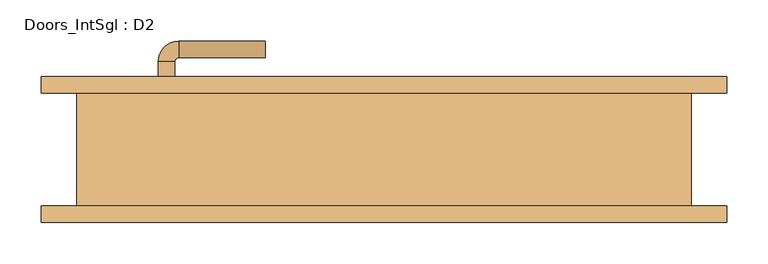
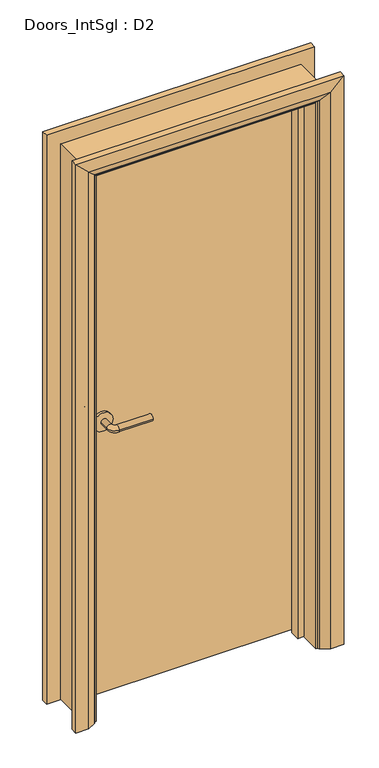
"""IFC4 building model written with IfcOpenShell, lengths in millimetres: door geometry, Doors_IntSgl : D2."""

from ifc_helpers import new_model, si_unit, point, frame, frame_2d, origin, place, context, project, spatial, polyline, circle_curve, ellipse_curve, trimmed, segment, composite_curve, outline, extrude, faceted_brep, source, transform, mapped, element, save
from ifc_brep_helpers import plane_surface, cylinder_surface, revolved_surface, advanced_brep


def doors_intsgl_d2_4a296642(model_context):
    return source(origin(), model_context, "Body", "SolidModel", [
        advanced_brep(
        [(-274.0, 22.58, 900.0), (-254.0, 22.58, 900.0), (-254.0, -7.42, 900.0), (-274.0, -7.42, 900.0), (-249.0, -12.42, 900.0), (-249.0, -32.42, 900.0), (-144.0, -32.42, 900.0), (-144.0, -12.42, 900.0)],
        [
            (0, 1, circle_curve(frame((-264.0, 22.58, 900.0), z_axis=(0.0, 1.0, 0.0), x_axis=(1.0, 0.0, 0.0)), 10.0)),
            (1, 0, circle_curve(frame((-264.0, 22.58, 900.0), z_axis=(0.0, 1.0, 0.0), x_axis=(1.0, 0.0, 0.0)), 10.0)),
            (1, 2),
            (2, 3, circle_curve(frame((-264.0, -7.42, 900.0), z_axis=(0.0, 1.0, 0.0), x_axis=(1.0, 0.0, 0.0)), 10.0)),
            (3, 0),
            (3, 2, circle_curve(frame((-264.0, -7.42, 900.0), z_axis=(0.0, 1.0, 0.0), x_axis=(1.0, 0.0, 0.0)), 10.0)),
            (4, 5, circle_curve(frame((-249.0, -22.42, 900.0), z_axis=(-1.0, 0.0, 0.0), x_axis=(0.0, 1.0, 0.0)), 10.0)),
            (5, 3, circle_curve(frame((-249.0, -7.42, 900.0), z_axis=(0.0, 0.0, -1.0), x_axis=(-1.0, 0.0, 0.0)), 25.0)),
            (2, 4, circle_curve(frame((-249.0, -7.42, 900.0), z_axis=(0.0, 0.0, 1.0), x_axis=(-1.0, 0.0, 0.0)), 5.0)),
            (5, 4, circle_curve(frame((-249.0, -22.42, 900.0), z_axis=(-1.0, 0.0, 0.0), x_axis=(0.0, 1.0, 0.0)), 10.0)),
            (6, 7, circle_curve(frame((-144.0, -22.42, 900.0), z_axis=(1.0, 0.0, 0.0), x_axis=(0.0, 1.0, 0.0)), 10.0)),
            (7, 6, circle_curve(frame((-144.0, -22.42, 900.0), z_axis=(1.0, 0.0, 0.0), x_axis=(0.0, 1.0, 0.0)), 10.0)),
            (4, 7),
            (6, 5),
        ],
        [
            plane_surface(frame((-264.0, 22.58, 900.0), z_axis=(0.0, 1.0, 0.0), x_axis=(0.0, 0.0, 1.0))),
            cylinder_surface(frame((-264.0, 22.58, 900.0), z_axis=(0.0, 1.0, 0.0), x_axis=(1.0, 0.0, 0.0)), 10.0),
            revolved_surface(trimmed(ellipse_curve(frame((-264.0, -7.42, 900.0), z_axis=(0.0, -1.0, 0.0), x_axis=(1.0, 0.0, 0.0)), 10.0, 10.0), [point((-274.0, -7.42, 900.0))], [point((-254.0, -7.42, 900.0))], True, "CARTESIAN"), (-249.0, -7.42, 900.0), (0.0, 0.0, -1.0)),
            revolved_surface(trimmed(ellipse_curve(frame((-264.0, -7.42, 900.0), z_axis=(0.0, -1.0, 0.0), x_axis=(1.0, 0.0, 0.0)), 10.0, 10.0), [point((-254.0, -7.42, 900.0))], [point((-274.0, -7.42, 900.0))], True, "CARTESIAN"), (-249.0, -7.42, 900.0), (0.0, 0.0, -1.0)),
            plane_surface(frame((-144.0, -22.42, 900.0), z_axis=(1.0, 0.0, 0.0), x_axis=(0.0, 0.0, 1.0))),
            cylinder_surface(frame((-249.0, -22.42, 900.0), z_axis=(-1.0, 0.0, 0.0), x_axis=(0.0, 1.0, 0.0)), 10.0),
        ],
        [
            (0, [[1, 2]]),
            (1, [[3, 4, 5, -2]]),
            (1, [[-5, 6, -3, -1]]),
            (2, [[7, 8, -4, 9]]),
            (3, [[10, -9, -6, -8]]),
            (4, [[11, 12]]),
            (5, [[13, -11, 14, -7]]),
            (5, [[-14, -12, -13, -10]]),
        ],
    ),
        extrude(outline(composite_curve([segment(trimmed(circle_curve(frame_2d((900.0, -266.5)), 30.0), [point((900.0, -296.5))], [point((900.0, -236.5))], False, "CARTESIAN"), True, "CONTINUOUS"), segment(trimmed(circle_curve(frame_2d((900.0, -266.5)), 30.0), [point((900.0, -236.5))], [point((900.0, -296.5))], False, "CARTESIAN"), True, "CONTINUOUS")], self_intersect=False)), frame((0.0, 22.58, 0.0), z_axis=(0.0, 1.0, 0.0), x_axis=(0.0, 0.0, 1.0)), (0.0, 0.0, 1.0), 8.0),
        advanced_brep(
        [(-274.0, 76.58, 900.0), (-254.0, 76.58, 900.0), (-274.0, 106.58, 900.0), (-254.0, 106.58, 900.0), (-249.0, 111.58, 900.0), (-249.0, 131.58, 900.0), (-144.0, 131.58, 900.0), (-144.0, 111.58, 900.0)],
        [
            (0, 1, circle_curve(frame((-264.0, 76.58, 900.0), z_axis=(0.0, -1.0, 0.0), x_axis=(1.0, 0.0, 0.0)), 10.0)),
            (1, 0, circle_curve(frame((-264.0, 76.58, 900.0), z_axis=(0.0, -1.0, 0.0), x_axis=(1.0, 0.0, 0.0)), 10.0)),
            (0, 2),
            (2, 3, circle_curve(frame((-264.0, 106.58, 900.0), z_axis=(0.0, -1.0, 0.0), x_axis=(1.0, 0.0, 0.0)), 10.0)),
            (3, 1),
            (3, 2, circle_curve(frame((-264.0, 106.58, 900.0), z_axis=(0.0, -1.0, 0.0), x_axis=(1.0, 0.0, 0.0)), 10.0)),
            (4, 3, circle_curve(frame((-249.0, 106.58, 900.0), z_axis=(0.0, 0.0, 1.0), x_axis=(-1.0, 0.0, 0.0)), 5.0)),
            (2, 5, circle_curve(frame((-249.0, 106.58, 900.0), z_axis=(0.0, 0.0, -1.0), x_axis=(-1.0, 0.0, 0.0)), 25.0)),
            (5, 4, circle_curve(frame((-249.0, 121.58, 900.0), z_axis=(-1.0, 0.0, 0.0), x_axis=(0.0, -1.0, 0.0)), 10.0)),
            (4, 5, circle_curve(frame((-249.0, 121.58, 900.0), z_axis=(-1.0, 0.0, 0.0), x_axis=(0.0, -1.0, 0.0)), 10.0)),
            (6, 7, circle_curve(frame((-144.0, 121.58, 900.0), z_axis=(1.0, 0.0, 0.0), x_axis=(0.0, -1.0, 0.0)), 10.0)),
            (7, 6, circle_curve(frame((-144.0, 121.58, 900.0), z_axis=(1.0, 0.0, 0.0), x_axis=(0.0, -1.0, 0.0)), 10.0)),
            (5, 6),
            (7, 4),
        ],
        [
            plane_surface(frame((-264.0, 76.58, 900.0), z_axis=(0.0, -1.0, 0.0), x_axis=(0.0, 0.0, 1.0))),
            cylinder_surface(frame((-264.0, 76.58, 900.0), z_axis=(0.0, -1.0, 0.0), x_axis=(1.0, 0.0, 0.0)), 10.0),
            revolved_surface(trimmed(ellipse_curve(frame((-264.0, 106.58, 900.0), z_axis=(0.0, -1.0, 0.0), x_axis=(1.0, 0.0, 0.0)), 10.0, 10.0), [point((-274.0, 106.58, 900.0))], [point((-254.0, 106.58, 900.0))], True, "CARTESIAN"), (-249.0, 106.58, 900.0), (0.0, 0.0, -1.0)),
            revolved_surface(trimmed(ellipse_curve(frame((-264.0, 106.58, 900.0), z_axis=(0.0, -1.0, 0.0), x_axis=(1.0, 0.0, 0.0)), 10.0, 10.0), [point((-254.0, 106.58, 900.0))], [point((-274.0, 106.58, 900.0))], True, "CARTESIAN"), (-249.0, 106.58, 900.0), (0.0, 0.0, -1.0)),
            plane_surface(frame((-144.0, 121.58, 900.0), z_axis=(1.0, 0.0, 0.0), x_axis=(0.0, 0.0, 1.0))),
            cylinder_surface(frame((-249.0, 121.58, 900.0), z_axis=(-1.0, 0.0, 0.0), x_axis=(0.0, -1.0, 0.0)), 10.0),
        ],
        [
            (0, [[1, 2]]),
            (1, [[-1, 3, 4, 5]]),
            (1, [[-2, -5, 6, -3]]),
            (2, [[7, -4, 8, 9]]),
            (3, [[-8, -6, -7, 10]]),
            (4, [[11, 12]]),
            (5, [[-9, 13, -12, 14]]),
            (5, [[-10, -14, -11, -13]]),
        ],
    ),
        extrude(outline(composite_curve([segment(trimmed(circle_curve(frame_2d((900.0, -266.5)), 30.0), [point((900.0, -296.5))], [point((900.0, -236.5))], False, "CARTESIAN"), True, "CONTINUOUS"), segment(trimmed(circle_curve(frame_2d((900.0, -266.5)), 30.0), [point((900.0, -236.5))], [point((900.0, -296.5))], False, "CARTESIAN"), True, "CONTINUOUS")], self_intersect=False)), frame((0.0, 68.58, 0.0), z_axis=(0.0, 1.0, 0.0), x_axis=(0.0, 0.0, 1.0)), (0.0, 0.0, 1.0), 8.0),
        extrude(outline(polyline([(339.0, 30.58), (-339.0, 30.58), (-339.0, 68.58), (339.0, 68.58), (339.0, 30.58)])), frame((0.0, 0.0, 8.0), z_axis=(0.0, 0.0, 1.0), x_axis=(1.0, 0.0, 0.0)), (0.0, 0.0, 1.0), 1778.8),
        advanced_brep(
        [(416.0, 88.58, 0.0), (416.0, 68.58, 0.0), (346.0, 68.58, 0.0), (350.0, 74.58, 0.0), (376.0, 88.58, 0.0), (416.0, 88.58, 1863.8), (416.0, 68.58, 1863.8), (-416.0, 68.58, 1863.8), (-416.0, 68.58, 0.0), (-346.0, 68.58, 0.0), (-346.0, 68.58, 1793.8), (346.0, 68.58, 1793.8), (350.0, 74.58, 1797.8), (376.0, 88.58, 1823.8), (-376.0, 88.58, 1823.8), (-376.0, 88.58, 0.0), (-416.0, 88.58, 0.0), (-416.0, 88.58, 1863.8), (-350.0, 74.58, 0.0), (-350.0, 74.58, 1797.8)],
        [
            (0, 1),
            (1, 2),
            (2, 3, circle_curve(frame((354.0, 67.58, 0.0), z_axis=(0.0, 0.0, -1.0), x_axis=(1.0, 0.0, 0.0)), 8.0622577)),
            (3, 4),
            (4, 0),
            (0, 5),
            (5, 6),
            (6, 1),
            (6, 7),
            (7, 8),
            (8, 9),
            (9, 10),
            (10, 11),
            (11, 2),
            (11, 12, ellipse_curve(frame((354.0, 67.58, 1801.8), z_axis=(0.7071067811865475, 0.0, -0.7071067811865475), x_axis=(-0.7071067811865474, 0.0, -0.7071067811865476)), 11.4017543, 8.0622577)),
            (12, 3),
            (12, 13),
            (13, 4),
            (13, 14),
            (14, 15),
            (15, 16),
            (16, 17),
            (17, 5),
            (7, 17),
            (16, 8),
            (15, 18),
            (18, 9, circle_curve(frame((-354.0, 67.58, 0.0), z_axis=(0.0, 0.0, -1.0), x_axis=(-1.0, 0.0, 0.0)), 8.0622577)),
            (19, 10, ellipse_curve(frame((-354.0, 67.58, 1801.8), z_axis=(-0.7071067811865475, 0.0, -0.7071067811865475), x_axis=(-0.7071067811865474, 0.0, 0.7071067811865476)), 11.4017543, 8.0622577)),
            (18, 19),
            (14, 19),
            (19, 12),
        ],
        [
            plane_surface(frame((346.0, 68.58, 0.0), z_axis=(0.0, 0.0, -1.0), x_axis=(0.0, -1.0, 0.0))),
            plane_surface(frame((416.0, 88.58, 0.0), z_axis=(1.0, 0.0, 0.0), x_axis=(0.0, 0.0, 1.0))),
            plane_surface(frame((416.0, 68.58, 0.0), z_axis=(0.0, -1.0, 0.0), x_axis=(0.0, 0.0, 1.0))),
            cylinder_surface(frame((354.0, 67.58, 0.0), z_axis=(0.0, 0.0, -1.0), x_axis=(1.0, 0.0, 0.0)), 8.0622577),
            plane_surface(frame((350.0, 74.58, 0.0), z_axis=(-0.4740998230350126, 0.880471099922178, 0.0), x_axis=(0.0, 0.0, 1.0))),
            plane_surface(frame((376.0, 88.58, 0.0), z_axis=(0.0, 1.0, 0.0), x_axis=(0.0, 0.0, 1.0))),
            plane_surface(frame((-416.0, 88.58, 1863.8), z_axis=(-1.0, 0.0, 0.0), x_axis=(0.0, 0.0, -1.0))),
            plane_surface(frame((-346.0, 68.58, 0.0), z_axis=(0.0, 0.0, -1.0), x_axis=(0.0, -1.0, 0.0))),
            cylinder_surface(frame((-354.0, 67.58, 1793.8), z_axis=(0.0, 0.0, 1.0), x_axis=(-1.0, 0.0, 0.0)), 8.0622577),
            plane_surface(frame((-350.0, 74.58, 1797.8), z_axis=(0.47409982303501824, 0.8804710999221749, 0.0), x_axis=(0.0, 0.0, -1.0))),
            plane_surface(frame((416.0, 88.58, 1863.8), z_axis=(0.0, 0.0, 1.0), x_axis=(-1.0, 0.0, 0.0))),
            cylinder_surface(frame((346.0, 67.58, 1801.8), z_axis=(1.0, 0.0, 0.0), x_axis=(0.0, 0.0, 1.0)), 8.0622577),
            plane_surface(frame((350.0, 74.58, 1797.8), z_axis=(0.0, 0.8804710999221764, -0.4740998230350154), x_axis=(-1.0, 0.0, 0.0))),
        ],
        [
            (0, [[1, 2, 3, 4, 5]]),
            (1, [[-1, 6, 7, 8]]),
            (2, [[-2, -8, 9, 10, 11, 12, 13, 14]]),
            (3, [[-3, -14, 15, 16]]),
            (4, [[-4, -16, 17, 18]]),
            (5, [[-5, -18, 19, 20, 21, 22, 23, -6]]),
            (6, [[24, -22, 25, -10]]),
            (7, [[-21, 26, 27, -11, -25]]),
            (8, [[28, -12, -27, 29]]),
            (9, [[30, -29, -26, -20]]),
            (10, [[-7, -23, -24, -9]]),
            (11, [[-15, -13, -28, 31]]),
            (12, [[-17, -31, -30, -19]]),
        ],
    ),
        extrude(outline(polyline([(0.0, -341.0), (0.0, -322.0), (1769.8, -322.0), (1769.8, 322.0), (0.0, 322.0), (0.0, 341.0), (1788.8, 341.0), (1788.8, -341.0), (0.0, -341.0)])), frame((0.0, -3.42, 0.0), z_axis=(0.0, 1.0, 0.0), x_axis=(0.0, 0.0, 1.0)), (0.0, 0.0, 1.0), 32.0),
        advanced_brep(
        [(-416.0, -88.58, 0.0), (-416.0, -68.58, 0.0), (-346.0, -68.58, 0.0), (-350.0, -74.58, 0.0), (-376.0, -88.58, 0.0), (-416.0, -88.58, 1863.8), (-416.0, -68.58, 1863.8), (-346.0, -68.58, 1793.8), (-350.0, -74.58, 1797.8), (-376.0, -88.58, 1823.8), (416.0, -88.58, 0.0), (376.0, -88.58, 0.0), (350.0, -74.58, 0.0), (346.0, -68.58, 0.0), (416.0, -68.58, 0.0), (416.0, -88.58, 1863.8), (376.0, -88.58, 1823.8), (350.0, -74.58, 1797.8), (346.0, -68.58, 1793.8), (416.0, -68.58, 1863.8)],
        [
            (0, 1),
            (1, 2),
            (2, 3, circle_curve(frame((-354.0, -67.58, 0.0), z_axis=(0.0, 0.0, -1.0), x_axis=(-1.0, 0.0, 0.0)), 8.0622577)),
            (3, 4),
            (4, 0),
            (0, 5),
            (5, 6),
            (6, 1),
            (6, 7),
            (7, 2),
            (7, 8, ellipse_curve(frame((-354.0, -67.58, 1801.8), z_axis=(-0.7071067811865475, 0.0, -0.7071067811865475), x_axis=(0.7071067811865474, 0.0, -0.7071067811865476)), 11.4017543, 8.0622577)),
            (8, 3),
            (8, 9),
            (9, 4),
            (9, 5),
            (10, 11),
            (11, 12),
            (12, 13, circle_curve(frame((354.0, -67.58, 0.0), z_axis=(0.0, 0.0, -1.0), x_axis=(1.0, 0.0, 0.0)), 8.0622577)),
            (13, 14),
            (14, 10),
            (15, 16),
            (16, 11),
            (10, 15),
            (16, 17),
            (17, 12),
            (17, 18, ellipse_curve(frame((354.0, -67.58, 1801.8), z_axis=(0.7071067811865475, 0.0, -0.7071067811865475), x_axis=(0.7071067811865474, 0.0, 0.7071067811865476)), 11.4017543, 8.0622577)),
            (18, 13),
            (18, 19),
            (19, 14),
            (19, 15),
            (5, 15),
            (19, 6),
            (18, 7),
            (17, 8),
            (16, 9),
        ],
        [
            plane_surface(frame((-346.0, -141.3810989, 0.0), z_axis=(0.0, 0.0, -1.0), x_axis=(1.0, 0.0, 0.0))),
            plane_surface(frame((-416.0, -88.58, 0.0), z_axis=(-1.0, 0.0, 0.0), x_axis=(0.0, 0.0, 1.0))),
            plane_surface(frame((-416.0, -68.58, 0.0), z_axis=(0.0, 1.0, 0.0), x_axis=(0.0, 0.0, 1.0))),
            cylinder_surface(frame((-354.0, -67.58, 0.0), z_axis=(0.0, 0.0, -1.0), x_axis=(-1.0, 0.0, 0.0)), 8.0622577),
            plane_surface(frame((-350.0, -74.58, 0.0), z_axis=(0.4740998230350183, -0.8804710999221749, 0.0), x_axis=(0.0, 0.0, 1.0))),
            plane_surface(frame((-376.0, -88.58, 0.0), z_axis=(0.0, -1.0, 0.0), x_axis=(0.0, 0.0, 1.0))),
            plane_surface(frame((346.0, -141.3810989, 0.0), z_axis=(0.0, 0.0, -1.0), x_axis=(-1.0, 0.0, 0.0))),
            plane_surface(frame((376.0, -88.58, 1823.8), z_axis=(0.0, -1.0, 0.0), x_axis=(0.0, 0.0, -1.0))),
            plane_surface(frame((350.0, -74.58, 1797.8), z_axis=(-0.4740998230350183, -0.8804710999221749, 0.0), x_axis=(0.0, 0.0, -1.0))),
            cylinder_surface(frame((354.0, -67.58, 1793.8), z_axis=(0.0, 0.0, 1.0), x_axis=(1.0, 0.0, 0.0)), 8.0622577),
            plane_surface(frame((416.0, -68.58, 1863.8), z_axis=(0.0, 1.0, 0.0), x_axis=(0.0, 0.0, -1.0))),
            plane_surface(frame((416.0, -88.58, 1863.8), z_axis=(1.0, 0.0, 0.0), x_axis=(0.0, 0.0, -1.0))),
            plane_surface(frame((-416.0, -88.58, 1863.8), z_axis=(0.0, 0.0, 1.0), x_axis=(1.0, 0.0, 0.0))),
            plane_surface(frame((-416.0, -68.58, 1863.8), z_axis=(0.0, 1.0, 0.0), x_axis=(1.0, 0.0, 0.0))),
            cylinder_surface(frame((-346.0, -67.58, 1801.8), z_axis=(-1.0, 0.0, 0.0), x_axis=(0.0, 0.0, 1.0)), 8.0622577),
            plane_surface(frame((-350.0, -74.58, 1797.8), z_axis=(0.0, -0.8804710999221749, -0.4740998230350183), x_axis=(1.0, 0.0, 0.0))),
            plane_surface(frame((-376.0, -88.58, 1823.8), z_axis=(0.0, -1.0, 0.0), x_axis=(1.0, 0.0, 0.0))),
        ],
        [
            (0, [[1, 2, 3, 4, 5]]),
            (1, [[-1, 6, 7, 8]]),
            (2, [[-2, -8, 9, 10]]),
            (3, [[-3, -10, 11, 12]]),
            (4, [[-4, -12, 13, 14]]),
            (5, [[-5, -14, 15, -6]]),
            (6, [[16, 17, 18, 19, 20]]),
            (7, [[21, 22, -16, 23]]),
            (8, [[24, 25, -17, -22]]),
            (9, [[26, 27, -18, -25]]),
            (10, [[28, 29, -19, -27]]),
            (11, [[30, -23, -20, -29]]),
            (12, [[-7, 31, -30, 32]]),
            (13, [[-9, -32, -28, 33]]),
            (14, [[-11, -33, -26, 34]]),
            (15, [[-13, -34, -24, 35]]),
            (16, [[-15, -35, -21, -31]]),
        ],
    ),
        faceted_brep([(-341.0, 68.58, 0.0), (-341.0, -68.58, 0.0), (-373.0, -68.58, 0.0), (-373.0, 68.58, 0.0), (-341.0, 68.58, 1788.8), (-341.0, -68.58, 1788.8), (-373.0, -68.58, 1820.8), (-373.0, 68.58, 1820.8), (341.0, 68.58, 0.0), (373.0, 68.58, 0.0), (373.0, -68.58, 0.0), (341.0, -68.58, 0.0), (341.0, 68.58, 1788.8), (373.0, 68.58, 1820.8), (373.0, -68.58, 1820.8), (341.0, -68.58, 1788.8)], [[[0, 1, 2, 3]], [[1, 0, 4, 5]], [[2, 1, 5, 6]], [[3, 2, 6, 7]], [[0, 3, 7, 4]], [[8, 9, 10, 11]], [[12, 13, 9, 8]], [[13, 14, 10, 9]], [[14, 15, 11, 10]], [[15, 12, 8, 11]], [[5, 4, 12, 15]], [[6, 5, 15, 14]], [[7, 6, 14, 13]], [[4, 7, 13, 12]]]),
    ])


if __name__ == "__main__":
    model = new_model("IFC4")
    model_context = context("Model", 3, world=origin())
    ifc_project = project(units=[si_unit("LENGTHUNIT", "METRE", prefix="MILLI")], contexts=[model_context])
    site = spatial("IfcSite", under=ifc_project)
    building = spatial("IfcBuilding", under=site)
    placement = place(None, origin())
    doors_intsgl_d2_shape = doors_intsgl_d2_4a296642(model_context)
    element("IfcDoor", 1, ObjectType="Doors_IntSgl : D2", at=placement, inside=building, context=model_context, shape_type="MappedRepresentation", body=[
        mapped(doors_intsgl_d2_shape, transform((0.0, 0.0, 0.0), x_axis=(1.0, 0.0, 0.0), y_axis=(0.0, 1.0, 0.0), z_axis=(0.0, 0.0, 1.0))),
    ])
    save(model, "model.ifc")

# Revit data of these elements
# Type "Doors_IntSgl : D2"
#   Type Mark = "47"
#   Type Comments = "Internal Single"
#   Operation = "SingleSwingRight"
#   Manufacturer = "Revit"
#   Keynote = "L20"
#   Description = "Internal Single Door"
#   Analytic Construction = "Metal"
#   UnderCut = 0.026247 ft
#   Tolerance = 0.006562 ft
#   Thickness = 0.124672 ft
#   Thermal Resistance (R) = 0.270117 (m²·K)/W
#   Structural Tolerance = 0.026247 ft
#   StopDepth = 0.104987 ft
#   Stop Thickness = 0.062336 ft
#   Rough Width = 2.5 ft
#   Rough Height = 6.0 ft
#   Height to Top Lock Rail = 3.28084 ft
#   Heat Transfer Coefficient (U) = 3.7021 W/(m²·K)
#   Handle Z Distance = 2.952756 ft
#   Handle X Distance = 0.246063 ft
#   Frame Thickness = 0.104987 ft
#   Door Panel Width = 2.224409 ft
#   Door Panel Thickness = 0.124672 ft
#   Door Panel Offset = 0.0 ft
#   Height = 6.0 ft
#   Width = 2.5 ft
#   Door Panel Height = 5.835958 ft
#   Architrave Setback = 0.016404 ft
#   Vis - Ironmongery = yes
#   Material Ironmongery = Door - Handle
#   Material Frame = Door - Frame/Mullion (1)
#   Material Door = Door - Panel
#   Material Architrave = Door - Architrave
#   Visual Light Transmittance = 0
#   Solar Heat Gain Coefficient = 0
#   Function = (empty or 0)
#   Wall Closure = (empty or 0)
# Element 1 (IfcDoor, "Doors_IntSgl : D2")
#   Materials on its faces: "Door - Architrave", "Door - Handle", "Door - Frame/Mullion (1)", "Door - Panel"
# Materials
#   "Door - Handle": colour RGB 0 0 0, transparency 0, Keynote = "P21", Cost = 0
#   "Door - Frame/Mullion (1)": class "Wood", colour RGB 212 179 113, transparency 0, Keynote = "L20", Cost = 0
#   "Door - Panel": class "Wood", colour RGB 210 159 95, transparency 0, Keynote = "L20", Cost = 0
#   "Door - Architrave": class "Wood", colour RGB 154 90 5, transparency 0, Keynote = "P20", Cost = 0
